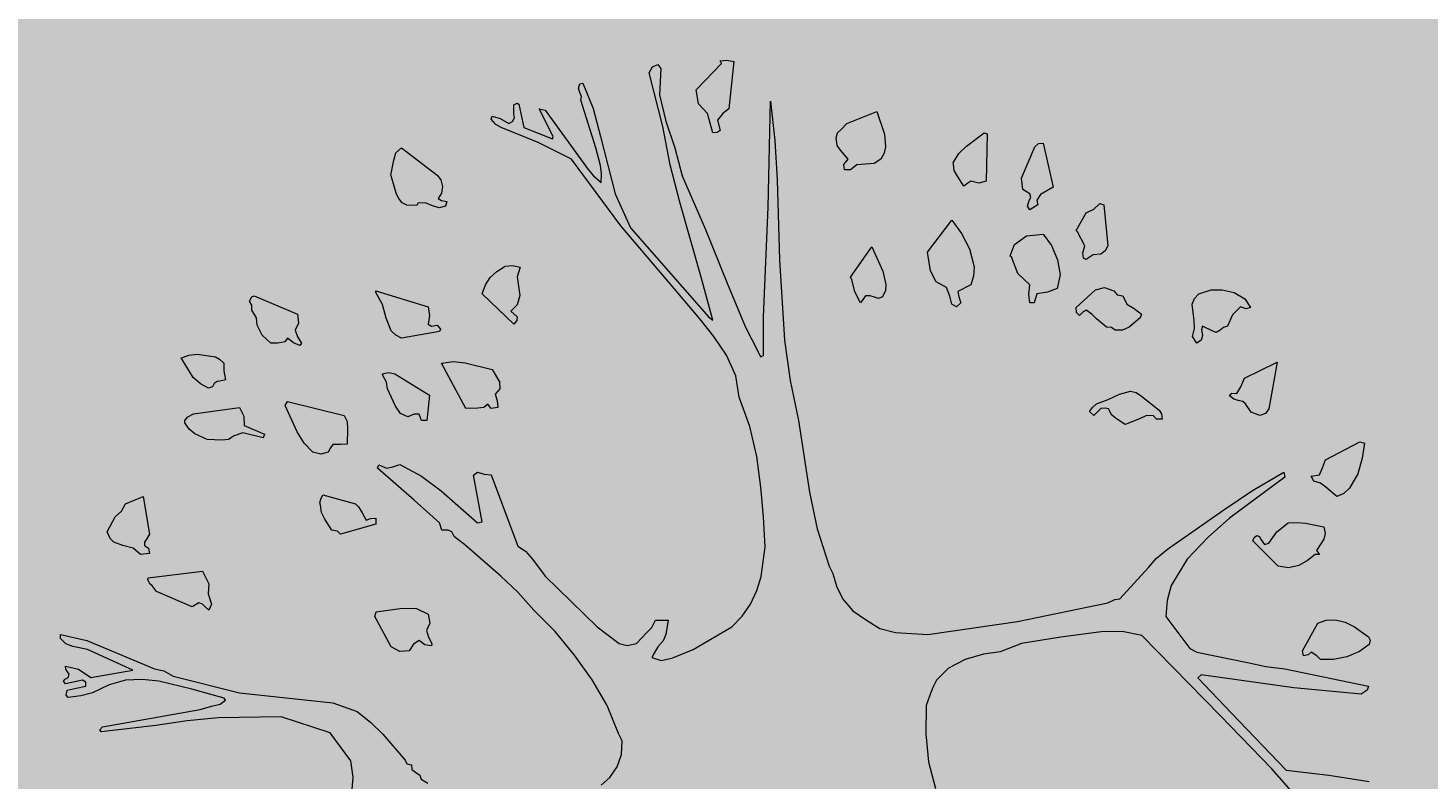
# Model space of a CAD drawing. Units: inches. Extents: x 84 to 1044, y -280 to 906.
# Tile 55 of 105: x 389.11 to 411.62, y 726.41 to 738.5. Entities that reach past the tile are written whole.
import ezdxf

# ---------------------------------------------------------------- set-up
doc = ezdxf.new("R2010")
doc.units = ezdxf.units.IN
doc.layers.add('A-ANNO-DIMS', color=2, linetype='Continuous', lineweight=18)
doc.layers.add('L-PLNT', color=114, linetype='Continuous', lineweight=15)
doc.layers.add('L-PLNT-PATT', color=9, linetype='Continuous', lineweight=9, true_color=0xafd9aa)
doc.styles.get("Standard").update_dxf_attribs({"font": 'arial.ttf'})
doc.dimstyles.get("Standard").update_dxf_attribs({"dimtxt": 0.18, "dimasz": 0.18, "dimexe": 0.18, "dimexo": 0.0625, "dimgap": 0.09, "dimtad": 0, "dimtih": 1, "dimtoh": 1, "dimdec": 4, "dimzin": 0, "dimdsep": 46, "dimtxsty": 'Standard', "dimcen": 0.09, "dimadec": 0, "dimazin": 0, "dimtfac": 1, "dimtdec": 4, "dimtofl": 0, "dimtmove": 0, "dimatfit": 3, "dimfxl": 1, "dimtolj": 1, "dimtzin": 0, "dimarcsym": 0})

# ---------------------------------------------------------------- blocks, each defined once
blk = doc.blocks.new('A$C37E508DF')
for p, q in [((0.6329, 1.5111), (0.6367, 1.5175)), ((0.6475, 1.4545), (0.6329, 1.5111)), ((0.6367, 1.5175), (0.6423, 1.5201)), ((0.6423, 1.5201), (0.6453, 1.5158)), ((0.6453, 1.5158), (0.644, 1.4879)), ((0.6826, 1.493), (0.7096, 1.5209)), ((0.7083, 1.5239), (0.7152, 1.5244)), ((0.7096, 1.5209), (0.7083, 1.5239)), ((0.7152, 1.5244), (0.7225, 1.5231)), ((0.7225, 1.5231), (0.7174, 1.4729)), ((0.5583, 1.4948), (0.5596, 1.4995)), ((0.5596, 1.4995), (0.563, 1.5003)), ((0.563, 1.5003), (0.5737, 1.4733)), ((0.5596, 1.4905), (0.5583, 1.4948)), ((0.5613, 1.4862), (0.5596, 1.4905)), ((0.5608, 1.4823), (0.5613, 1.4862)), ((0.5767, 1.4317), (0.5608, 1.4823)), ((0.644, 1.4879), (0.6505, 1.46)), ((0.6852, 1.4785), (0.6826, 1.493)), ((0.4897, 1.4772), (0.4935, 1.4789)), ((0.4897, 1.4678), (0.4897, 1.4772)), ((0.4905, 1.4635), (0.4897, 1.4678)), ((0.4935, 1.4789), (0.4952, 1.478)), ((0.4952, 1.478), (0.5004, 1.4532)), ((0.5313, 1.4437), (0.5167, 1.4729)), ((0.5167, 1.4729), (0.5231, 1.4716)), ((0.5231, 1.4716), (0.5686, 1.409)), ((0.5737, 1.4733), (0.5814, 1.4437)), ((0.6946, 1.4682), (0.6852, 1.4785)), ((0.6976, 1.4579), (0.6946, 1.4682)), ((0.7109, 1.4682), (0.7053, 1.4609)), ((0.7174, 1.4729), (0.7109, 1.4682)), ((0.7589, 1.3691), (0.7615, 1.481)), ((0.7615, 1.481), (0.7658, 1.4395)), ((0.8421, 1.4575), (0.8739, 1.4703)), ((0.8739, 1.4703), (0.882, 1.4463)), ((0.4657, 1.4622), (0.4669, 1.4652)), ((0.4708, 1.4566), (0.4657, 1.4622)), ((0.4669, 1.4652), (0.4755, 1.463)), ((0.4764, 1.4532), (0.4708, 1.4566)), ((0.4755, 1.463), (0.4845, 1.4575)), ((0.5154, 1.4373), (0.4764, 1.4532)), ((0.4845, 1.4575), (0.4884, 1.4596)), ((0.4884, 1.4596), (0.4905, 1.4635)), ((0.5004, 1.4532), (0.5308, 1.4412)), ((0.6552, 1.4137), (0.6475, 1.4545)), ((0.6505, 1.46), (0.6603, 1.4317)), ((0.7002, 1.4476), (0.6976, 1.4579)), ((0.7053, 1.4609), (0.7083, 1.4502)), ((0.8357, 1.451), (0.8421, 1.4575)), ((0.551, 1.4197), (0.5154, 1.4373)), ((0.5308, 1.4412), (0.5313, 1.4437)), ((0.5814, 1.4437), (0.5969, 1.3833)), ((0.7049, 1.448), (0.7002, 1.4476)), ((0.7083, 1.4502), (0.7049, 1.448)), ((0.7658, 1.4395), (0.7684, 1.3979)), ((0.831, 1.4424), (0.8323, 1.4476)), ((0.8318, 1.4343), (0.831, 1.4424)), ((0.8323, 1.4476), (0.8357, 1.451)), ((0.882, 1.4463), (0.8829, 1.433)), ((0.9686, 1.4334), (0.9875, 1.4476)), ((0.9875, 1.4476), (0.9905, 1.4467)), ((0.9905, 1.4467), (0.9896, 1.3966)), ((1.045, 1.4365), (1.0497, 1.4369)), ((1.0497, 1.4369), (1.0604, 1.3901)), ((0.3628, 1.4189), (0.3649, 1.4266)), ((0.3649, 1.4266), (0.3709, 1.4317)), ((0.3709, 1.4317), (0.4086, 1.403)), ((0.5814, 1.4133), (0.5767, 1.4317)), ((0.6603, 1.4317), (0.668, 1.4021)), ((0.8353, 1.4292), (0.8318, 1.4343)), ((0.8434, 1.4197), (0.8353, 1.4292)), ((0.8816, 1.4262), (0.8781, 1.4197)), ((0.8829, 1.433), (0.8816, 1.4262)), ((0.9545, 1.4159), (0.9605, 1.4257)), ((0.9605, 1.4257), (0.9686, 1.4334)), ((1.0269, 1.3996), (1.0411, 1.433)), ((1.0411, 1.433), (1.045, 1.4365)), ((0.3598, 1.403), (0.3628, 1.4189)), ((0.6029, 1.3494), (0.551, 1.4197)), ((0.5686, 1.409), (0.5741, 1.4021)), ((0.5827, 1.4043), (0.5814, 1.4133)), ((0.6655, 1.3743), (0.6552, 1.4137)), ((0.8391, 1.4141), (0.8434, 1.4197)), ((0.8395, 1.4086), (0.8391, 1.4141)), ((0.846, 1.4086), (0.8395, 1.4086)), ((0.8528, 1.4137), (0.846, 1.4086)), ((0.8619, 1.4146), (0.8528, 1.4137)), ((0.8709, 1.4154), (0.8619, 1.4146)), ((0.8781, 1.4197), (0.8709, 1.4154)), ((0.9549, 1.4146), (0.9545, 1.4159)), ((0.9558, 1.4077), (0.9549, 1.4146)), ((0.9592, 1.4017), (0.9558, 1.4077)), ((0.3602, 1.4021), (0.3598, 1.403)), ((0.364, 1.3888), (0.3602, 1.4021)), ((0.4086, 1.403), (0.4125, 1.3979)), ((0.4125, 1.3979), (0.4142, 1.391)), ((0.5741, 1.4021), (0.5823, 1.3953)), ((0.5823, 1.3953), (0.5827, 1.4043)), ((0.668, 1.4021), (0.6925, 1.3455)), ((0.7684, 1.3979), (0.771, 1.3134)), ((0.966, 1.3914), (0.9592, 1.4017)), ((0.9703, 1.3944), (0.966, 1.3914)), ((0.9733, 1.3966), (0.9703, 1.3944)), ((0.9819, 1.3944), (0.9733, 1.3966)), ((0.9896, 1.3966), (0.9819, 1.3944)), ((1.0282, 1.3876), (1.0269, 1.3996)), ((0.3657, 1.3828), (0.364, 1.3888)), ((0.3683, 1.3781), (0.3657, 1.3828)), ((0.3718, 1.3738), (0.3683, 1.3781)), ((0.4134, 1.3837), (0.4099, 1.3781)), ((0.4099, 1.3781), (0.4134, 1.376)), ((0.4142, 1.391), (0.4134, 1.3837)), ((0.5969, 1.3833), (0.6132, 1.3472)), ((1.0359, 1.3833), (1.0282, 1.3876)), ((1.0351, 1.376), (1.0368, 1.3794)), ((1.0368, 1.3794), (1.0359, 1.3833)), ((1.0471, 1.3824), (1.0432, 1.3764)), ((1.0604, 1.3901), (1.0471, 1.3824)), ((0.3765, 1.3713), (0.3718, 1.3738)), ((0.3872, 1.3708), (0.3765, 1.3713)), ((0.3885, 1.3738), (0.3872, 1.3708)), ((0.3971, 1.3734), (0.3885, 1.3738)), ((0.4039, 1.3704), (0.3971, 1.3734)), ((0.4108, 1.3683), (0.4039, 1.3704)), ((0.4176, 1.37), (0.4108, 1.3683)), ((0.4134, 1.376), (0.4189, 1.3751)), ((0.4189, 1.3751), (0.4176, 1.37)), ((0.6882, 1.2949), (0.6655, 1.3743)), ((0.7538, 1.2529), (0.7589, 1.3691)), ((1.0334, 1.37), (1.0351, 1.376)), ((1.0359, 1.3661), (1.0334, 1.37)), ((1.0441, 1.3717), (1.0359, 1.3661)), ((1.0432, 1.3764), (1.0441, 1.3717)), ((1.0848, 1.3443), (1.0955, 1.3631)), ((1.0955, 1.3631), (1.1033, 1.367)), ((1.1033, 1.367), (1.1097, 1.373)), ((1.1097, 1.373), (1.114, 1.3717)), ((1.114, 1.3717), (1.1183, 1.328)), ((0.6595, 1.2829), (0.6029, 1.3494)), ((0.9274, 1.3215), (0.9532, 1.3554)), ((0.9532, 1.3554), (0.9635, 1.3413)), ((0.6132, 1.3472), (0.6959, 1.2529)), ((0.6925, 1.3455), (0.7161, 1.2868)), ((0.9635, 1.3413), (0.9721, 1.325)), ((1.0197, 1.3297), (1.0321, 1.3387)), ((1.0321, 1.3387), (1.0497, 1.3404)), ((1.0497, 1.3404), (1.0587, 1.3284)), ((1.0861, 1.343), (1.0848, 1.3443)), ((1.0938, 1.328), (1.0861, 1.343)), ((0.846, 1.2949), (0.8687, 1.3271)), ((0.8687, 1.3271), (0.8803, 1.3014)), ((0.9279, 1.3194), (0.9274, 1.3215)), ((0.9305, 1.3018), (0.9279, 1.3194)), ((0.9721, 1.325), (0.9768, 1.3061)), ((1.0149, 1.3172), (1.0171, 1.3232)), ((1.0171, 1.3232), (1.0197, 1.3297)), ((1.0587, 1.3284), (1.0651, 1.3134)), ((1.0917, 1.3207), (1.0938, 1.328)), ((1.0925, 1.3151), (1.0917, 1.3207)), ((1.1028, 1.3185), (1.0955, 1.3138)), ((1.111, 1.3194), (1.1028, 1.3185)), ((1.1153, 1.3228), (1.111, 1.3194)), ((1.1183, 1.328), (1.1153, 1.3228)), ((0.4717, 1.3009), (0.4807, 1.3065)), ((0.4807, 1.3065), (0.4884, 1.3074)), ((0.4884, 1.3074), (0.4965, 1.3057)), ((0.4965, 1.3057), (0.4935, 1.2954)), ((0.771, 1.3134), (0.7761, 1.2285)), ((0.9768, 1.3061), (0.9763, 1.2962)), ((1.0162, 1.3164), (1.0149, 1.3172)), ((1.0231, 1.2988), (1.0162, 1.3164)), ((1.0651, 1.3134), (1.0677, 1.2975)), ((1.0955, 1.3138), (1.0925, 1.3151)), ((0.4597, 1.2868), (0.4648, 1.2945)), ((0.4648, 1.2945), (0.4717, 1.3009)), ((0.4935, 1.2954), (0.4948, 1.2855)), ((0.7002, 1.2495), (0.6882, 1.2949)), ((0.8473, 1.2924), (0.846, 1.2949)), ((0.8507, 1.2795), (0.8473, 1.2924)), ((0.8803, 1.3014), (0.8833, 1.2872)), ((0.9365, 1.2902), (0.9305, 1.3018)), ((0.9476, 1.2842), (0.9365, 1.2902)), ((0.9763, 1.2962), (0.9733, 1.2868)), ((1.0359, 1.2868), (1.0231, 1.2988)), ((1.0677, 1.2975), (1.0647, 1.2829)), ((0.2101, 1.2696), (0.2127, 1.2744)), ((0.2127, 1.2744), (0.2152, 1.2752)), ((0.2152, 1.2752), (0.2611, 1.2559)), ((0.3439, 1.2804), (0.3992, 1.2636)), ((0.3439, 1.2787), (0.3439, 1.2804)), ((0.3507, 1.2662), (0.3439, 1.2787)), ((0.4562, 1.2774), (0.4597, 1.2868)), ((0.4897, 1.2452), (0.4562, 1.2774)), ((0.4961, 1.2756), (0.4935, 1.2658)), ((0.4948, 1.2855), (0.4961, 1.2756)), ((0.6865, 1.2508), (0.6595, 1.2829)), ((0.7161, 1.2868), (0.7349, 1.2422)), ((0.8567, 1.2679), (0.8507, 1.2795)), ((0.8619, 1.2752), (0.8567, 1.2679)), ((0.867, 1.2752), (0.8619, 1.2752)), ((0.8713, 1.2739), (0.867, 1.2752)), ((0.8756, 1.2726), (0.8713, 1.2739)), ((0.8799, 1.2744), (0.8756, 1.2726)), ((0.8829, 1.2808), (0.8799, 1.2744)), ((0.8833, 1.2872), (0.8829, 1.2808)), ((0.951, 1.2748), (0.9476, 1.2842)), ((0.9532, 1.2666), (0.951, 1.2748)), ((0.9733, 1.2868), (0.9596, 1.2799)), ((0.9596, 1.2799), (0.9605, 1.2744)), ((0.9605, 1.2744), (0.9626, 1.2679)), ((1.0347, 1.2769), (1.0359, 1.2868)), ((1.0359, 1.2679), (1.0347, 1.2769)), ((1.0432, 1.2774), (1.0402, 1.2679)), ((1.0544, 1.2791), (1.0432, 1.2774)), ((1.0647, 1.2829), (1.0544, 1.2791)), ((1.0848, 1.2628), (1.1054, 1.2817)), ((1.1054, 1.2817), (1.1148, 1.2842)), ((1.1148, 1.2842), (1.1247, 1.2804)), ((1.1247, 1.2804), (1.1281, 1.2765)), ((1.1281, 1.2765), (1.1341, 1.2752)), ((1.1341, 1.2752), (1.1384, 1.2666)), ((1.21, 1.2726), (1.2147, 1.2774)), ((1.2147, 1.2774), (1.2276, 1.2817)), ((1.2276, 1.2817), (1.2392, 1.2817)), ((1.2392, 1.2817), (1.2521, 1.2787)), ((1.2521, 1.2787), (1.2632, 1.2722)), ((0.2127, 1.2654), (0.2101, 1.2696)), ((0.2127, 1.2602), (0.2127, 1.2654)), ((0.2174, 1.2521), (0.2127, 1.2602)), ((0.3546, 1.2516), (0.3507, 1.2662)), ((0.3992, 1.2636), (0.4005, 1.2546)), ((0.4935, 1.2658), (0.4867, 1.2589)), ((0.9583, 1.2636), (0.9532, 1.2666)), ((0.9626, 1.2679), (0.9583, 1.2636)), ((1.0402, 1.2679), (1.0359, 1.2679)), ((1.0852, 1.2576), (1.0848, 1.2628)), ((1.0955, 1.2602), (1.0921, 1.2585)), ((1.1015, 1.2559), (1.0955, 1.2602)), ((1.1384, 1.2666), (1.1461, 1.2619)), ((1.1461, 1.2619), (1.1539, 1.2559)), ((1.2075, 1.2666), (1.21, 1.2726)), ((1.2096, 1.2491), (1.2075, 1.2666)), ((1.2585, 1.2636), (1.2503, 1.2551)), ((1.2645, 1.2615), (1.2585, 1.2636)), ((1.2632, 1.2722), (1.2692, 1.2628)), ((1.2692, 1.2628), (1.2645, 1.2615)), ((0.2182, 1.2443), (0.2174, 1.2521)), ((0.2234, 1.2336), (0.2182, 1.2443)), ((0.262, 1.2465), (0.2586, 1.2388)), ((0.2611, 1.2559), (0.262, 1.2465)), ((0.3602, 1.2383), (0.3546, 1.2516)), ((0.4005, 1.2546), (0.3992, 1.2452)), ((0.3992, 1.2452), (0.4026, 1.2431)), ((0.4026, 1.2431), (0.4086, 1.2443)), ((0.4086, 1.2443), (0.4121, 1.2401)), ((0.4867, 1.2589), (0.4935, 1.2529)), ((0.4931, 1.2491), (0.4897, 1.2452)), ((0.4935, 1.2529), (0.4931, 1.2491)), ((0.7015, 1.2323), (0.6865, 1.2508)), ((0.6959, 1.2529), (0.7002, 1.2495)), ((0.7538, 1.2122), (0.7538, 1.2529)), ((1.0883, 1.2546), (1.0852, 1.2576)), ((1.0921, 1.2585), (1.0883, 1.2546)), ((1.1063, 1.2508), (1.1015, 1.2559)), ((1.117, 1.2422), (1.1063, 1.2508)), ((1.1526, 1.2521), (1.141, 1.2422)), ((1.1539, 1.2559), (1.1526, 1.2521)), ((1.21, 1.2409), (1.2096, 1.2491)), ((1.2503, 1.2551), (1.2448, 1.2431)), ((0.2328, 1.2251), (0.2234, 1.2336)), ((0.2504, 1.2306), (0.2474, 1.2268)), ((0.2568, 1.2255), (0.2504, 1.2306)), ((0.2586, 1.2388), (0.2611, 1.2319)), ((0.2611, 1.2319), (0.265, 1.2251)), ((0.3649, 1.2336), (0.3602, 1.2383)), ((0.3709, 1.2306), (0.3649, 1.2336)), ((0.4112, 1.2375), (0.3709, 1.2306)), ((0.4121, 1.2401), (0.4112, 1.2375)), ((0.7148, 1.2126), (0.7015, 1.2323)), ((0.7349, 1.2422), (0.7482, 1.216)), ((1.1221, 1.2418), (1.117, 1.2422)), ((1.126, 1.2388), (1.1221, 1.2418)), ((1.1337, 1.2388), (1.126, 1.2388)), ((1.141, 1.2422), (1.1337, 1.2388)), ((1.2079, 1.2323), (1.21, 1.2409)), ((1.2126, 1.2251), (1.2079, 1.2323)), ((1.2186, 1.2332), (1.2169, 1.2285)), ((1.2186, 1.2431), (1.2173, 1.2392)), ((1.2173, 1.2392), (1.2186, 1.2332)), ((1.2285, 1.2383), (1.2186, 1.2431)), ((1.2328, 1.2366), (1.2285, 1.2383)), ((1.2371, 1.2388), (1.2328, 1.2366)), ((1.2405, 1.2418), (1.2371, 1.2388)), ((1.2448, 1.2431), (1.2405, 1.2418)), ((0.2401, 1.2251), (0.2328, 1.2251)), ((0.2474, 1.2268), (0.2401, 1.2251)), ((0.2633, 1.2229), (0.2568, 1.2255)), ((0.265, 1.2251), (0.2633, 1.2229)), ((0.7482, 1.216), (0.7508, 1.2109)), ((0.7761, 1.2285), (0.7821, 1.1856)), ((1.2169, 1.2285), (1.2126, 1.2251)), ((0.1376, 1.2092), (0.1458, 1.2126)), ((0.1389, 1.2079), (0.1376, 1.2092)), ((0.1505, 1.189), (0.1389, 1.2079)), ((0.1458, 1.2126), (0.1548, 1.2135)), ((0.1548, 1.2135), (0.1741, 1.2109)), ((0.1741, 1.2109), (0.1784, 1.2083)), ((0.1784, 1.2083), (0.1831, 1.204)), ((0.1831, 1.204), (0.1831, 1.1959)), ((0.4134, 1.204), (0.4258, 1.2058)), ((0.4391, 1.156), (0.4134, 1.204)), ((0.4258, 1.2058), (0.4382, 1.2045)), ((0.4382, 1.2045), (0.4669, 1.1972)), ((0.7246, 1.1908), (0.7148, 1.2126)), ((0.7508, 1.2109), (0.7538, 1.2122)), ((1.2628, 1.1882), (1.2975, 1.2053)), ((1.2975, 1.2053), (1.2885, 1.1556)), ((0.1582, 1.1822), (0.1505, 1.189)), ((0.1788, 1.1852), (0.1758, 1.1847)), ((0.1848, 1.1865), (0.1788, 1.1852)), ((0.1831, 1.1959), (0.1848, 1.1865)), ((0.3507, 1.1916), (0.352, 1.1933)), ((0.355, 1.1839), (0.3507, 1.1916)), ((0.352, 1.1933), (0.3576, 1.1942)), ((0.3576, 1.1942), (0.364, 1.1929)), ((0.364, 1.1929), (0.4005, 1.1702)), ((0.4669, 1.1972), (0.4747, 1.1843)), ((0.7281, 1.168), (0.7246, 1.1908)), ((0.7821, 1.1856), (0.7911, 1.1436)), ((1.2589, 1.1792), (1.2628, 1.1882)), ((0.1668, 1.1775), (0.1582, 1.1822)), ((0.1711, 1.1792), (0.1668, 1.1775)), ((0.1728, 1.1826), (0.1711, 1.1792)), ((0.1758, 1.1847), (0.1728, 1.1826)), ((0.3563, 1.177), (0.355, 1.1839)), ((0.3645, 1.1586), (0.3563, 1.177)), ((0.4005, 1.1702), (0.3979, 1.1436)), ((0.4751, 1.177), (0.47, 1.1714)), ((0.47, 1.1714), (0.4721, 1.1646)), ((0.4747, 1.1843), (0.4751, 1.177)), ((1.1187, 1.1655), (1.1307, 1.1714)), ((1.1307, 1.1714), (1.1423, 1.1744)), ((1.1423, 1.1744), (1.1483, 1.1732)), ((1.1483, 1.1732), (1.1539, 1.1693)), ((1.2469, 1.1702), (1.2495, 1.1723)), ((1.2478, 1.1693), (1.2469, 1.1702)), ((1.2495, 1.1723), (1.2546, 1.1719)), ((1.2546, 1.1719), (1.2589, 1.1792)), ((0.1509, 1.1504), (0.1994, 1.1573)), ((0.1994, 1.1573), (0.2041, 1.1479)), ((0.2478, 1.1594), (0.2504, 1.1637)), ((0.2607, 1.1316), (0.2478, 1.1594)), ((0.2504, 1.1637), (0.3104, 1.1487)), ((0.37, 1.1509), (0.3645, 1.1586)), ((0.4519, 1.1564), (0.4391, 1.156)), ((0.458, 1.1573), (0.4519, 1.1564)), ((0.4622, 1.1607), (0.458, 1.1573)), ((0.4657, 1.156), (0.4622, 1.1607)), ((0.473, 1.1573), (0.4657, 1.156)), ((0.4721, 1.1646), (0.473, 1.1573)), ((0.7396, 1.1371), (0.7281, 1.168)), ((1.099, 1.153), (1.102, 1.1573)), ((1.102, 1.1573), (1.1063, 1.1612)), ((1.111, 1.156), (1.1033, 1.1487)), ((1.1063, 1.1612), (1.1187, 1.1655)), ((1.1153, 1.1564), (1.111, 1.156)), ((1.1191, 1.1556), (1.1153, 1.1564)), ((1.1226, 1.1492), (1.1191, 1.1556)), ((1.1539, 1.1693), (1.1727, 1.1543)), ((1.2516, 1.1659), (1.2478, 1.1693)), ((1.2563, 1.1646), (1.2516, 1.1659)), ((1.2611, 1.1637), (1.2563, 1.1646)), ((1.2641, 1.1612), (1.2611, 1.1637)), ((1.2701, 1.1522), (1.2641, 1.1612)), ((1.2885, 1.1556), (1.2851, 1.1509)), ((0.1419, 1.1436), (0.1449, 1.1474)), ((0.1419, 1.141), (0.1419, 1.1436)), ((0.1462, 1.1342), (0.1419, 1.141)), ((0.1449, 1.1474), (0.1509, 1.1504)), ((0.2041, 1.1479), (0.2045, 1.138)), ((0.3104, 1.1487), (0.3134, 1.1423)), ((0.3134, 1.1423), (0.3139, 1.1346)), ((0.3778, 1.1474), (0.37, 1.1509)), ((0.3842, 1.15), (0.3778, 1.1474)), ((0.3898, 1.15), (0.3842, 1.15)), ((0.3923, 1.1436), (0.3898, 1.15)), ((0.3979, 1.1436), (0.3923, 1.1436)), ((0.7911, 1.1436), (0.8027, 1.0677)), ((1.1033, 1.1487), (1.099, 1.153)), ((1.1273, 1.1453), (1.1226, 1.1492)), ((1.1367, 1.1393), (1.1273, 1.1453)), ((1.1517, 1.1453), (1.1367, 1.1393)), ((1.1586, 1.1483), (1.1517, 1.1453)), ((1.1663, 1.1487), (1.1586, 1.1483)), ((1.1697, 1.1449), (1.1663, 1.1487)), ((1.1757, 1.1449), (1.1697, 1.1449)), ((1.1727, 1.1543), (1.1749, 1.1504)), ((1.1749, 1.1504), (1.1757, 1.1449)), ((1.2791, 1.1487), (1.2701, 1.1522)), ((1.2851, 1.1509), (1.2791, 1.1487)), ((0.1522, 1.1294), (0.1462, 1.1342)), ((0.1655, 1.1234), (0.1522, 1.1294)), ((0.1938, 1.1273), (0.1878, 1.1234)), ((0.2032, 1.1303), (0.1938, 1.1273)), ((0.2247, 1.1251), (0.2032, 1.1303)), ((0.2045, 1.138), (0.226, 1.129)), ((0.226, 1.129), (0.2247, 1.1251)), ((0.268, 1.1196), (0.2607, 1.1316)), ((0.3139, 1.1346), (0.3134, 1.1183)), ((0.7469, 1.1054), (0.7396, 1.1371)), ((0.181, 1.1226), (0.1655, 1.1234)), ((0.1878, 1.1234), (0.181, 1.1226)), ((0.277, 1.1101), (0.268, 1.1196)), ((0.2959, 1.1144), (0.2933, 1.1101)), ((0.2984, 1.1179), (0.2959, 1.1144)), ((0.3066, 1.1179), (0.2984, 1.1179)), ((0.3134, 1.1183), (0.3066, 1.1179)), ((1.3485, 1.102), (1.385, 1.1209)), ((1.385, 1.1209), (1.3897, 1.1196)), ((1.3897, 1.1196), (1.3875, 1.1037)), ((0.2856, 1.108), (0.277, 1.1101)), ((0.2933, 1.1101), (0.2856, 1.108)), ((0.3456, 1.093), (0.3469, 1.0964)), ((0.3469, 1.0964), (0.355, 1.093)), ((0.3619, 1.0943), (0.3692, 1.0968)), ((0.3692, 1.0968), (0.3923, 1.0844)), ((0.7512, 1.0728), (0.7469, 1.1054)), ((1.3455, 1.0934), (1.3485, 1.102)), ((1.3875, 1.1037), (1.3828, 1.087)), ((0.3842, 1.0591), (0.3456, 1.093)), ((0.355, 1.093), (0.3619, 1.0943)), ((0.3923, 1.0844), (0.4129, 1.069)), ((0.4472, 1.0857), (0.4515, 1.0887)), ((0.4562, 1.0364), (0.4472, 1.0857)), ((0.4515, 1.0887), (0.4584, 1.0865)), ((0.4584, 1.0865), (0.4657, 1.0861)), ((0.4657, 1.0861), (0.4939, 1.0107)), ((1.3057, 1.0835), (1.2469, 1.0402)), ((1.2713, 1.0694), (1.3044, 1.0887)), ((1.3044, 1.0887), (1.3057, 1.0835)), ((1.3335, 1.0844), (1.3421, 1.0861)), ((1.3361, 1.0793), (1.3335, 1.0844)), ((1.3421, 1.0861), (1.3455, 1.0934)), ((1.3828, 1.087), (1.3738, 1.072)), ((0.4129, 1.069), (0.4515, 1.0351)), ((0.7538, 1.0415), (0.7512, 1.0728)), ((0.8027, 1.0677), (0.8108, 1.0287)), ((1.2409, 1.0488), (1.2713, 1.0694)), ((1.3434, 1.0771), (1.3361, 1.0793)), ((1.349, 1.0728), (1.3434, 1.0771)), ((1.3605, 1.063), (1.349, 1.0728)), ((1.3738, 1.072), (1.3678, 1.0664)), ((0.0746, 1.0475), (0.0789, 1.0552)), ((0.0789, 1.0552), (0.0978, 1.063)), ((0.0978, 1.063), (0.1042, 1.0231)), ((0.2847, 1.0565), (0.2856, 1.0604)), ((0.2851, 1.054), (0.2847, 1.0565)), ((0.2864, 1.0463), (0.2851, 1.054)), ((0.2856, 1.0604), (0.2877, 1.0647)), ((0.2877, 1.0647), (0.3224, 1.0552)), ((0.3224, 1.0552), (0.3255, 1.0522)), ((0.3255, 1.0522), (0.3293, 1.0458)), ((0.4112, 1.0351), (0.3842, 1.0591)), ((1.3678, 1.0664), (1.3605, 1.063)), ((0.0596, 1.0257), (0.0682, 1.0415)), ((0.0682, 1.0415), (0.0746, 1.0475)), ((0.2899, 1.039), (0.2864, 1.0463)), ((0.2972, 1.0274), (0.2899, 1.039)), ((0.3293, 1.0458), (0.3336, 1.0381)), ((0.3336, 1.0381), (0.3383, 1.0398)), ((0.3383, 1.0398), (0.3439, 1.0402)), ((0.3439, 1.0402), (0.3439, 1.0338)), ((0.7559, 1.0098), (0.7538, 1.0415)), ((1.1813, 1.0072), (1.2409, 1.0488)), ((1.2469, 1.0402), (1.2246, 1.0201)), ((0.0626, 1.0188), (0.0596, 1.0257)), ((0.1042, 1.0231), (0.1012, 1.018)), ((0.3032, 1.0265), (0.2972, 1.0274)), ((0.3066, 1.0231), (0.3032, 1.0265)), ((0.3439, 1.0338), (0.3066, 1.0231)), ((0.4138, 1.0274), (0.4112, 1.0351)), ((0.4202, 1.0274), (0.4138, 1.0274)), ((0.4241, 1.0257), (0.4202, 1.0274)), ((0.4267, 1.0209), (0.4241, 1.0257)), ((0.4515, 1.0351), (0.4562, 1.0364)), ((0.8108, 1.0287), (0.8233, 0.9892)), ((1.2885, 1.0136), (1.2971, 1.0257)), ((1.2971, 1.0257), (1.3091, 1.0351)), ((1.3091, 1.0351), (1.3185, 1.0355)), ((1.3185, 1.0355), (1.3275, 1.0347)), ((1.3275, 1.0347), (1.3468, 1.0308)), ((1.3468, 1.0308), (1.3481, 1.0239)), ((1.3481, 1.0239), (1.3468, 1.018)), ((0.0665, 1.0149), (0.0626, 1.0188)), ((0.0763, 1.0111), (0.0665, 1.0149)), ((0.087, 1.0085), (0.0763, 1.0111)), ((0.0948, 1.0016), (0.087, 1.0085)), ((0.1012, 1.018), (0.099, 1.0149)), ((0.099, 1.0149), (0.099, 1.0111)), ((0.099, 1.0111), (0.1033, 1.0085)), ((0.1033, 1.0085), (0.1042, 1.0029)), ((0.4305, 1.0175), (0.4267, 1.0209)), ((0.4378, 1.0124), (0.4305, 1.0175)), ((0.476, 0.9789), (0.4378, 1.0124)), ((0.4939, 1.0107), (0.5021, 1.0051)), ((0.7516, 0.9785), (0.7559, 1.0098)), ((1.2246, 1.0201), (1.2023, 0.9969)), ((1.2718, 1.0162), (1.2731, 1.0197)), ((1.2984, 0.9892), (1.2718, 1.0162)), ((1.2731, 1.0197), (1.2761, 1.0218)), ((1.2761, 1.0218), (1.2786, 1.0209)), ((1.2786, 1.0209), (1.2799, 1.0184)), ((1.2799, 1.0184), (1.2842, 1.0124)), ((1.2842, 1.0124), (1.2885, 1.0136)), ((1.3468, 1.018), (1.3391, 1.0059)), ((0.1042, 1.0029), (0.0948, 1.0016)), ((0.5021, 1.0051), (0.5094, 0.9969)), ((0.5094, 0.9969), (0.5231, 0.9789)), ((1.1612, 0.9879), (1.1693, 0.9974)), ((1.1693, 0.9974), (1.1813, 1.0072)), ((1.2023, 0.9969), (1.1852, 0.9691)), ((1.3297, 0.9952), (1.3202, 0.9901)), ((1.3378, 1.0016), (1.3297, 0.9952)), ((1.3421, 1.0016), (1.3378, 1.0016)), ((1.3391, 1.0059), (1.3421, 1.0016)), ((0.1029, 0.9772), (0.1604, 0.9841)), ((0.1604, 0.9841), (0.1672, 0.9708)), ((0.4939, 0.9618), (0.476, 0.9789)), ((0.5231, 0.9789), (0.578, 0.9253)), ((0.7469, 0.9635), (0.7516, 0.9785)), ((0.8233, 0.9892), (0.8275, 0.9815)), ((0.8275, 0.9815), (0.8314, 0.9673)), ((1.1311, 0.9549), (1.1612, 0.9879)), ((1.3095, 0.9875), (1.2984, 0.9892)), ((1.3202, 0.9901), (1.3095, 0.9875)), ((0.1025, 0.9751), (0.1029, 0.9772)), ((0.1046, 0.9708), (0.1025, 0.9751)), ((0.1076, 0.9682), (0.1046, 0.9708)), ((0.1119, 0.9626), (0.1076, 0.9682)), ((0.1672, 0.9708), (0.1664, 0.9601)), ((0.7401, 0.9493), (0.7469, 0.9635)), ((0.8314, 0.9673), (0.8383, 0.954)), ((1.1852, 0.9691), (1.1809, 0.9532)), ((0.1496, 0.9463), (0.1119, 0.9626)), ((0.1565, 0.9506), (0.1496, 0.9463)), ((0.1604, 0.9493), (0.1565, 0.9506)), ((0.1629, 0.9468), (0.1604, 0.9493)), ((0.1664, 0.9601), (0.1698, 0.9493)), ((0.1698, 0.9493), (0.1672, 0.9429)), ((0.5111, 0.9429), (0.4939, 0.9618)), ((0.7315, 0.9365), (0.7401, 0.9493)), ((0.8383, 0.954), (0.8486, 0.942)), ((1.0227, 0.9309), (1.1183, 0.9506)), ((1.1183, 0.9506), (1.1256, 0.954)), ((1.1256, 0.954), (1.1311, 0.9549)), ((1.1809, 0.9532), (1.1796, 0.936)), ((0.1672, 0.9429), (0.1629, 0.9468)), ((0.3426, 0.936), (0.3443, 0.9412)), ((0.3602, 0.9039), (0.3426, 0.936)), ((0.3443, 0.9412), (0.3722, 0.9451)), ((0.3722, 0.9451), (0.3868, 0.9446)), ((0.3868, 0.9446), (0.3992, 0.9386)), ((0.3992, 0.9386), (0.4009, 0.9292)), ((0.5334, 0.9202), (0.5111, 0.9429)), ((0.7203, 0.9253), (0.7315, 0.9365)), ((0.8486, 0.942), (0.8619, 0.933)), ((1.1796, 0.936), (1.2049, 0.9022)), ((0.4009, 0.9292), (0.3975, 0.9215)), ((0.3975, 0.9215), (0.3996, 0.9142)), ((0.554, 0.8953), (0.5334, 0.9202)), ((0.578, 0.9253), (0.6011, 0.9077)), ((0.6196, 0.9077), (0.6303, 0.9189)), ((0.6303, 0.9189), (0.6359, 0.9245)), ((0.6359, 0.9245), (0.6397, 0.9322)), ((0.6397, 0.9322), (0.653, 0.9322)), ((0.653, 0.9322), (0.6505, 0.9172)), ((0.6796, 0.9013), (0.7203, 0.9253)), ((0.8619, 0.933), (0.8769, 0.9236)), ((0.8769, 0.9236), (0.8936, 0.9193)), ((0.8936, 0.9193), (0.9279, 0.9172)), ((0.9279, 0.9172), (1.0227, 0.9309)), ((1.1114, 0.9198), (1.0685, 0.9142)), ((1.1333, 0.9202), (1.1114, 0.9198)), ((1.1543, 0.9159), (1.1333, 0.9202)), ((1.3241, 0.9), (1.3404, 0.9292)), ((1.3404, 0.9292), (1.3494, 0.9322)), ((1.3494, 0.9322), (1.3592, 0.9326)), ((1.3592, 0.9326), (1.3695, 0.93)), ((1.3695, 0.93), (1.3794, 0.9253)), ((1.3794, 0.9253), (1.394, 0.9146)), ((0.0103, 0.9129), (0.0103, 0.9172)), ((0.0103, 0.9172), (0.0382, 0.9107)), ((0.0159, 0.9073), (0.0103, 0.9129)), ((0.0232, 0.9043), (0.0159, 0.9073)), ((0.0386, 0.9013), (0.0232, 0.9043)), ((0.0382, 0.9107), (0.1098, 0.8807)), ((0.3692, 0.8992), (0.3602, 0.9039)), ((0.3838, 0.9069), (0.379, 0.9)), ((0.3898, 0.9107), (0.3838, 0.9069)), ((0.3958, 0.906), (0.3898, 0.9107)), ((0.4026, 0.9052), (0.3958, 0.906)), ((0.3996, 0.9142), (0.4031, 0.9077)), ((0.4031, 0.9077), (0.4026, 0.9052)), ((0.6011, 0.9077), (0.6097, 0.9056)), ((0.6097, 0.9056), (0.6196, 0.9077)), ((0.6423, 0.9039), (0.6384, 0.8974)), ((0.6479, 0.9103), (0.6423, 0.9039)), ((0.6505, 0.9172), (0.6479, 0.9103)), ((1.0269, 0.9077), (1.0042, 0.8987)), ((1.0685, 0.9142), (1.0269, 0.9077)), ((1.2371, 0.8314), (1.1543, 0.9159)), ((1.3948, 0.9065), (1.3846, 0.8992)), ((1.394, 0.9146), (1.3957, 0.9112)), ((1.3957, 0.9112), (1.3948, 0.9065)), ((0.0866, 0.8794), (0.0386, 0.9013)), ((0.379, 0.9), (0.3692, 0.8992)), ((0.5728, 0.8691), (0.554, 0.8953)), ((0.6384, 0.8974), (0.6359, 0.8927)), ((0.6359, 0.8927), (0.6457, 0.8897)), ((0.6457, 0.8897), (0.6569, 0.8919)), ((0.6569, 0.8919), (0.6796, 0.9013)), ((0.9673, 0.8906), (0.9498, 0.8816)), ((0.9866, 0.8962), (0.9673, 0.8906)), ((1.0042, 0.8987), (0.9866, 0.8962)), ((1.2049, 0.9022), (1.2126, 0.8983)), ((1.2126, 0.8983), (1.2662, 0.8876)), ((1.3254, 0.8944), (1.3241, 0.9)), ((1.3301, 0.8957), (1.3254, 0.8944)), ((1.3335, 0.8983), (1.3301, 0.8957)), ((1.3395, 0.8944), (1.3335, 0.8983)), ((1.3434, 0.8906), (1.3395, 0.8944)), ((1.3571, 0.8906), (1.3434, 0.8906)), ((1.3713, 0.8936), (1.3571, 0.8906)), ((1.3846, 0.8992), (1.3713, 0.8936)), ((0.0159, 0.8803), (0.0154, 0.8837)), ((0.0154, 0.8837), (0.0292, 0.8803)), ((0.0176, 0.8777), (0.0159, 0.8803)), ((0.0193, 0.8752), (0.0176, 0.8777)), ((0.0184, 0.8717), (0.0193, 0.8752)), ((0.0292, 0.8803), (0.0424, 0.8717)), ((0.0424, 0.8717), (0.0866, 0.8794)), ((0.1098, 0.8807), (0.1196, 0.8786)), ((0.1196, 0.8786), (0.1295, 0.873)), ((0.9498, 0.8816), (0.9369, 0.8687)), ((1.2169, 0.8743), (1.2135, 0.8713)), ((1.3151, 0.8606), (1.2169, 0.8743)), ((1.2662, 0.8876), (1.2855, 0.8833)), ((1.2855, 0.8833), (1.3057, 0.8807)), ((1.3057, 0.8807), (1.394, 0.8623)), ((0.0133, 0.8679), (0.015, 0.87)), ((0.0154, 0.8649), (0.0133, 0.8679)), ((0.015, 0.87), (0.0184, 0.8717)), ((0.0334, 0.8687), (0.0154, 0.8649)), ((0.0171, 0.8584), (0.0266, 0.8602)), ((0.0266, 0.8602), (0.0369, 0.8623)), ((0.0369, 0.8666), (0.0334, 0.8687)), ((0.0369, 0.8623), (0.0369, 0.8666)), ((0.0617, 0.864), (0.0442, 0.8554)), ((0.0789, 0.8687), (0.0617, 0.864)), ((0.0965, 0.8696), (0.0789, 0.8687)), ((0.1141, 0.8679), (0.0965, 0.8696)), ((0.1492, 0.8593), (0.1141, 0.8679)), ((0.1295, 0.873), (0.1994, 0.8554)), ((0.1835, 0.8499), (0.1492, 0.8593)), ((0.5887, 0.8421), (0.5728, 0.8691)), ((0.933, 0.861), (0.9296, 0.852)), ((0.9369, 0.8687), (0.933, 0.861)), ((1.2135, 0.8713), (1.2491, 0.834)), ((1.3863, 0.8541), (1.3151, 0.8606)), ((1.394, 0.8623), (1.3927, 0.8584)), ((0.0163, 0.8529), (0.0171, 0.8584)), ((0.0184, 0.8503), (0.0163, 0.8529)), ((0.0317, 0.8524), (0.0184, 0.8503)), ((0.0442, 0.8554), (0.0317, 0.8524)), ((0.1792, 0.8434), (0.1848, 0.8477)), ((0.1848, 0.8477), (0.1835, 0.8499)), ((0.1994, 0.8554), (0.2984, 0.8447)), ((0.2984, 0.8447), (0.3242, 0.8357)), ((0.9296, 0.852), (0.9262, 0.8421)), ((1.3927, 0.8584), (1.3863, 0.8541)), ((0.0545, 0.8194), (0.1578, 0.8378)), ((0.1578, 0.8378), (0.1698, 0.8413)), ((0.1698, 0.8413), (0.1792, 0.8434)), ((0.2436, 0.8301), (0.1771, 0.8288)), ((0.2954, 0.813), (0.2436, 0.8301)), ((0.3242, 0.8357), (0.3387, 0.8241)), ((0.6007, 0.8125), (0.5887, 0.8421)), ((0.9262, 0.8421), (0.9257, 0.8121)), ((1.2919, 0.7752), (1.2371, 0.8314)), ((1.2491, 0.834), (1.3069, 0.7735)), ((0.0519, 0.8164), (0.0545, 0.8194)), ((0.0532, 0.8143), (0.0519, 0.8164)), ((0.1111, 0.8207), (0.0532, 0.8143)), ((0.1441, 0.8258), (0.1111, 0.8207)), ((0.1771, 0.8288), (0.1441, 0.8258)), ((0.3387, 0.8241), (0.3512, 0.8117)), ((0.3173, 0.7834), (0.2954, 0.813)), ((0.3512, 0.8117), (0.3748, 0.7842)), ((0.6046, 0.8048), (0.6007, 0.8125)), ((0.6037, 0.7903), (0.6046, 0.8048)), ((0.9257, 0.8121), (0.9287, 0.7825)), ((0.599, 0.777), (0.6037, 0.7903)), ((0.3199, 0.7662), (0.3173, 0.7834)), ((0.3748, 0.7842), (0.3765, 0.7804)), ((0.3765, 0.7804), (0.3816, 0.7791)), ((0.3816, 0.7791), (0.382, 0.7744)), ((0.382, 0.7744), (0.3859, 0.7714)), ((0.3859, 0.7714), (0.3902, 0.7684)), ((0.5913, 0.7658), (0.599, 0.777)), ((0.9287, 0.7825), (0.936, 0.7542)), ((1.3151, 0.7487), (1.2919, 0.7752)), ((1.3069, 0.7735), (1.352, 0.7684)), ((0.3186, 0.7491), (0.3199, 0.7662)), ((0.3902, 0.7684), (0.3919, 0.7641)), ((0.3919, 0.7641), (0.3988, 0.7598)), ((0.5823, 0.7577), (0.5913, 0.7658)), ((1.352, 0.7684), (1.3948, 0.7615))]:
    blk.add_line(p, q)
blk = doc.blocks.new('*D62')
at = {"layer": 'A-ANNO-DIMS', "color": 0, "lineweight": -2, "transparency": 16777216}
for p, q in [((203.179, 709.183), (203.179, 905.9)), ((896.074, 400.183), (896.074, 905.9)), ((203.359, 905.72), (549.232, 905.72)), ((895.894, 905.72), (550.021, 905.72))]:
    blk.add_line(p, q, dxfattribs=at)
at = {"layer": 'A-ANNO-DIMS', "color": 0, "transparency": 16777216}
for points in [[(203.359, 905.75), (203.359, 905.69), (203.179, 905.72)], [(895.894, 905.75), (895.894, 905.69), (896.074, 905.72)]]:
    blk.add_solid(points, dxfattribs=at)
at = {"layer": 'Defpoints', "color": 0, "transparency": 16777216}
for p in [(896.074, 905.72), (203.179, 709.12), (896.074, 400.12)]:
    blk.add_point(p, dxfattribs=at)
at = {"layer": 'A-ANNO-DIMS', "color": 0, "transparency": 16777216, "insert": (549.627, 905.72), "char_height": 0.18, "attachment_point": 5}
blk.add_mtext('\\A1;692.9', dxfattribs=at)

msp = doc.modelspace()

# ---------------------------------------------------------------- hatches: boundary and pattern name
at = {"layer": 'L-PLNT-PATT', "transparency": 33554597}
h = msp.add_hatch(color=256, dxfattribs=at)
h.dxf.hatch_style = 1
h.paths.add_polyline_path([(434.074, 769.12), (386.074, 769.12), (386.074, 709.12), (434.074, 709.12)])
h.paths.add_polyline_path([(896.074, 847.12), (434.074, 847.12), (434.074, 769.12), (434.074, 709.12), (470.074, 709.12), (506.074, 709.12), (572.074, 709.12), (608.074, 709.12), (698.074, 709.12), (770.074, 709.12), (833.074, 709.12), (896.074, 709.12)])
h.paths.add_polyline_path([(983.074, 847.12), (896.074, 847.12), (896.074, 709.12), (896.074, 547.12), (932.074, 547.12), (983.074, 547.12)])
h.paths.add_polyline_path([(983.074, 547.12), (932.074, 547.12), (932.074, 265.12), (983.074, 265.12)])
h.paths.add_polyline_path([(203.179, 646.12), (203.179, 709.12), (203.179, 745.12), (143.179, 745.12), (143.179, 271.12), (203.179, 271.12), (203.179, 274.12), (203.179, 310.12), (203.179, 574.12)])

# ---------------------------------------------------------------- block references
at = {"layer": 'L-PLNT', "xscale": 15.19586232982809, "yscale": 15.19586232982809, "zscale": 15.19586232982809}
msp.add_blockref('A$C37E508DF', (389.477, 714.812), dxfattribs=at)

# ---------------------------------------------------------------- dimensions: what is measured, and where the dimension line sits
at = {"layer": 'A-ANNO-DIMS'}
dim = msp.add_linear_dim(base=(896.074, 905.72), p1=(203.179, 709.12), p2=(896.074, 400.12), dimstyle='Standard', override={"dimdec": 1, "dimlfac": 1, "dimrnd": 0, "dimzin": 0, "dimdsep": 46, "dimlunit": 2}, dxfattribs=at)
dim.commit()
dim.dimension.update_dxf_attribs({"geometry": '*D62', "text_midpoint": (549.627, 905.72)})

doc.saveas('drawing.dxf')
